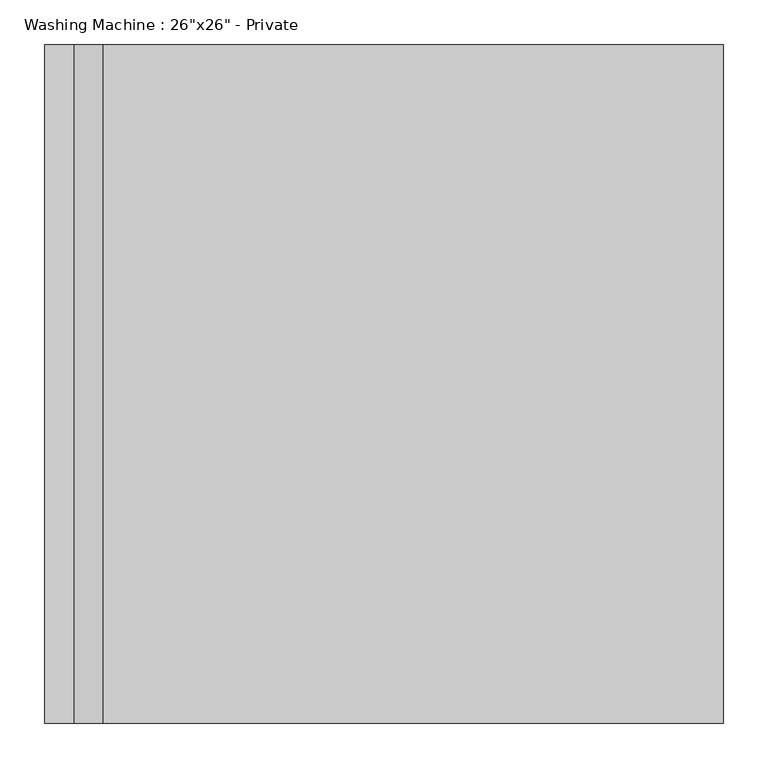
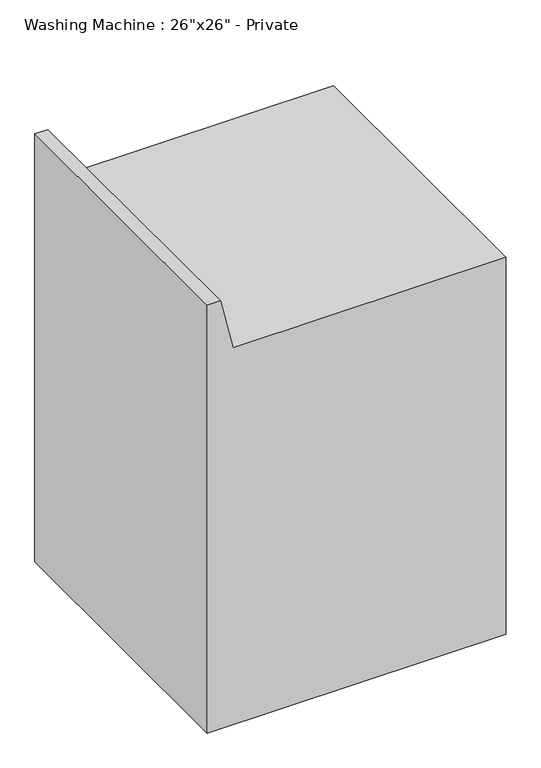
"""IFC4 building model written with IfcOpenShell, lengths in millimetres: flow terminal geometry."""

from ifc_helpers import new_model, si_unit, frame, origin, place, context, project, spatial, polyline, outline, extrude, source, transform, mapped, element, save


def flow_terminal_2ef58978(model_context):
    return source(origin(), model_context, "Body", "SweptSolid", [
        extrude(outline(polyline([(0.0, 762.0), (1016.0, 762.0), (1016.0, 65.88125), (1153.31875, 33.3375), (1153.31875, 0.0), (0.0, 0.0), (0.0, 762.0)])), frame((0.0, -381.0, 0.0), z_axis=(0.0, 1.0, 0.0), x_axis=(0.0, 0.0, 1.0)), (0.0, 0.0, 1.0), 762.0),
    ])


if __name__ == "__main__":
    model = new_model("IFC4")
    model_context = context("Model", 3, world=origin())
    ifc_project = project(units=[si_unit("LENGTHUNIT", "METRE", prefix="MILLI")], contexts=[model_context])
    site = spatial("IfcSite", under=ifc_project)
    building = spatial("IfcBuilding", under=site)
    placement = place(None, origin())
    flow_terminal_shape = flow_terminal_2ef58978(model_context)
    element("IfcFlowTerminal", 1, ObjectType="Washing Machine : 26\"x26\" - Private", at=placement, inside=building, context=model_context, shape_type="MappedRepresentation", body=[
        mapped(flow_terminal_shape, transform((0.0, 0.0, 0.0), x_axis=(1.0, 0.0, 0.0), y_axis=(0.0, 1.0, 0.0), z_axis=(0.0, 0.0, 1.0))),
    ])
    save(model, "model.ifc")

# Revit data of these elements
# Type "Washing Machine : 26\"x26\" - Private"
#   Sanitary Radius = 25.4 mm
#   Sanitary Diameter = 50.8 mm
#   Washing Machine Width = 2' - 6"
#   Washing Machine Length = 2' - 6"
#   Washing Machine Height = 3' - 4"
#   WFU = 2
#   Voltage = 120 V
#   Hot Water Radius = 12.7 mm
#   Hot Water Diameter = 25.4 mm
#   Half Washing Machine Width = 1' - 3"
#   HWFU = 1
#   Flow Pressure [instance default] = 55158.1 Pa
#   Cold Water Radius = 12.7 mm
#   Cold Water Diameter = 25.4 mm
#   CWFU = 1
#   Apparent Load = 600 VA
#   Number of Poles = 1
#   Washing Machine Material = none
#   Default Elevation = 0
#   Assembly Code = ""
